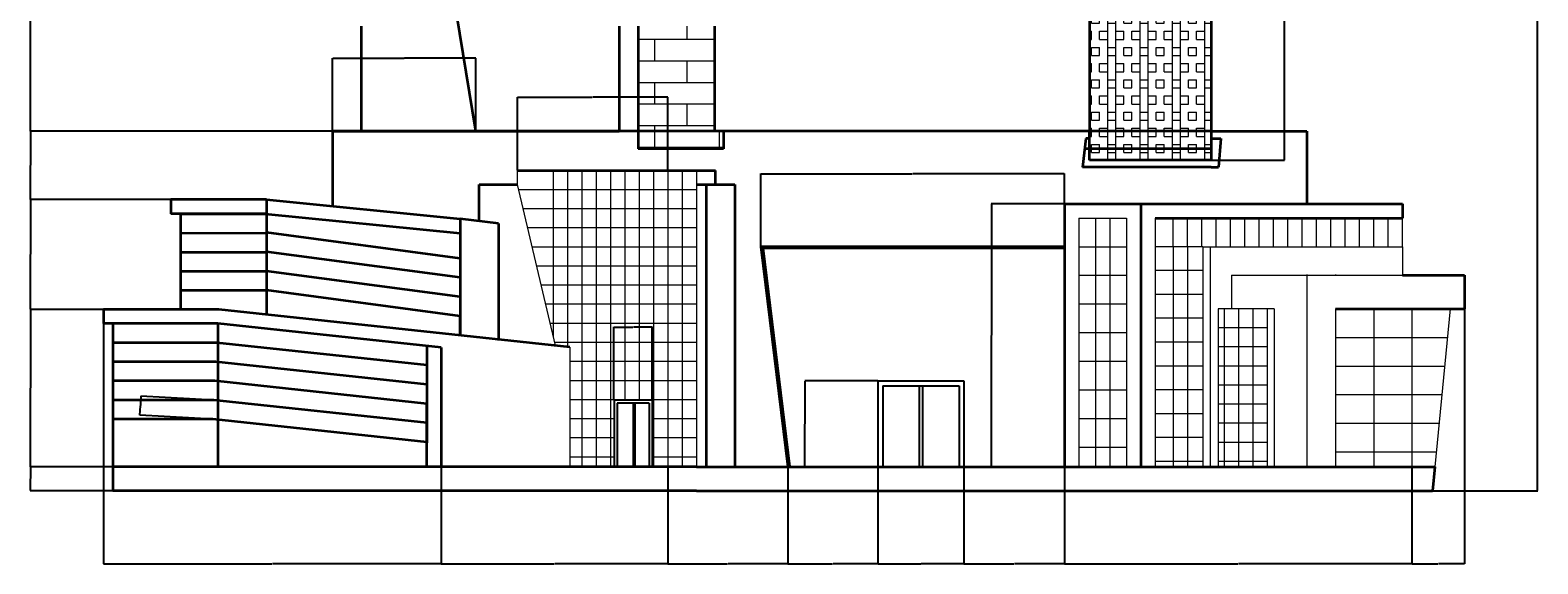
# Model space of a CAD drawing. Units: inches. Extents: x 597 to 2491, y 560 to 2558.
# Tile 1 of 2: x 597 to 2491, y 560 to 1231. Entities that reach past the tile are written whole.
import ezdxf

# ---------------------------------------------------------------- set-up
doc = ezdxf.new("R2010")
doc.units = ezdxf.units.IN
for name, color, linetype, lineweight in [('A-ANNO-DIMS', 2, 'Continuous', 18), ('A-DOOR', 3, 'Continuous', 25), ('A-ELEV', 7, 'Continuous', 35), ('A-ELEV-PATT', 8, 'Continuous', 13), ('A-GLAZ', 4, 'Continuous', 18)]:
    doc.layers.add(name, color=color, linetype=linetype, lineweight=lineweight)
doc.styles.get("Standard").update_dxf_attribs({"font": 'arial.ttf'})
doc.dimstyles.get("Standard").update_dxf_attribs({"dimtxt": 0.18, "dimasz": 0.18, "dimexe": 0.18, "dimexo": 0.0625, "dimgap": 0.09, "dimtad": 0, "dimtih": 1, "dimtoh": 1, "dimdec": 4, "dimzin": 0, "dimdsep": 46, "dimtxsty": 'Standard', "dimcen": 0.09, "dimadec": 0, "dimazin": 0, "dimtfac": 1, "dimtdec": 4, "dimtofl": 0, "dimtmove": 0, "dimatfit": 3, "dimfxl": 1, "dimtolj": 1, "dimtzin": 0, "dimarcsym": 0})

# ---------------------------------------------------------------- blocks, each defined once
blk = doc.blocks.new('*D1')
at = {"layer": 'A-ANNO-DIMS', "color": 0, "lineweight": -2, "transparency": 16777216}
for p, q in [((1478.3, 2465.8), (2491, 2465.8)), ((2490.9, 2465.6), (2490.9, 1559)), ((2490.9, 652.1), (2490.9, 1558.7)), ((701.1, 651.9), (2491, 651.9))]:
    blk.add_line(p, q, dxfattribs=at)
at = {"layer": 'A-ANNO-DIMS', "color": 0, "transparency": 16777216}
for points in [[(2490.8, 2465.6), (2490.9, 2465.6), (2490.9, 2465.8)], [(2490.8, 652.1), (2490.9, 652.1), (2490.9, 651.9)]]:
    blk.add_solid(points, dxfattribs=at)
at = {"layer": 'Defpoints', "color": 0, "transparency": 16777216}
for p in [(1478.2, 2465.8), (2490.9, 2465.8), (701, 651.9)]:
    blk.add_point(p, dxfattribs=at)
at = {"layer": 'A-ANNO-DIMS', "color": 0, "transparency": 16777216, "insert": (2490.9, 1558.9), "char_height": 0.18, "attachment_point": 5}
blk.add_mtext('\\A1;1814', dxfattribs=at)
blk = doc.blocks.new('*D2')
at = {"layer": 'A-ANNO-DIMS', "color": 0, "lineweight": -2, "transparency": 16777216}
for p, q in [((689, 861.9), (689, 560)), ((1113.3, 681.4), (1113.3, 560)), ((689.2, 560.2), (900.8, 560.2)), ((1113.1, 560.2), (901.6, 560.2))]:
    blk.add_line(p, q, dxfattribs=at)
at = {"layer": 'A-ANNO-DIMS', "color": 0, "transparency": 16777216}
for points in [[(689.2, 560.2), (689.2, 560.1), (689, 560.2)], [(1113.1, 560.2), (1113.1, 560.1), (1113.3, 560.2)]]:
    blk.add_solid(points, dxfattribs=at)
at = {"layer": 'Defpoints', "color": 0, "transparency": 16777216}
for p in [(689, 861.9), (1113.3, 681.5), (1113.3, 560.2)]:
    blk.add_point(p, dxfattribs=at)
at = {"layer": 'A-ANNO-DIMS', "color": 0, "transparency": 16777216, "insert": (901.2, 560.2), "char_height": 0.18, "attachment_point": 5}
blk.add_mtext('\\A1;424.2', dxfattribs=at)
blk = doc.blocks.new('*D3')
at = {"layer": 'A-ANNO-DIMS', "color": 0, "lineweight": -2, "transparency": 16777216}
for p, q in [((1113.3, 681.4), (1113.3, 560)), ((1398.1, 681.9), (1398.1, 560)), ((1113.4, 560.2), (1255.2, 560.2)), ((1398, 560.2), (1256.2, 560.2))]:
    blk.add_line(p, q, dxfattribs=at)
at = {"layer": 'A-ANNO-DIMS', "color": 0, "transparency": 16777216}
for points in [[(1113.4, 560.2), (1113.4, 560.1), (1113.3, 560.2)], [(1398, 560.2), (1398, 560.1), (1398.1, 560.2)]]:
    blk.add_solid(points, dxfattribs=at)
at = {"layer": 'Defpoints', "color": 0, "transparency": 16777216}
for p in [(1398.1, 681.9), (1113.3, 681.5), (1398.1, 560.2)]:
    blk.add_point(p, dxfattribs=at)
at = {"layer": 'A-ANNO-DIMS', "color": 0, "transparency": 16777216, "insert": (1255.7, 560.2), "char_height": 0.18, "attachment_point": 5}
blk.add_mtext('\\A1;284.87', dxfattribs=at)
blk = doc.blocks.new('*D4')
at = {"layer": 'A-ANNO-DIMS', "color": 0, "lineweight": -2, "transparency": 16777216}
for p, q in [((1398.1, 681.9), (1398.1, 560)), ((1548.9, 681.9), (1548.9, 560)), ((1398.3, 560.2), (1473.2, 560.2)), ((1548.8, 560.2), (1473.9, 560.2))]:
    blk.add_line(p, q, dxfattribs=at)
at = {"layer": 'A-ANNO-DIMS', "color": 0, "transparency": 16777216}
for points in [[(1398.3, 560.2), (1398.3, 560.1), (1398.1, 560.2)], [(1548.8, 560.2), (1548.8, 560.1), (1548.9, 560.2)]]:
    blk.add_solid(points, dxfattribs=at)
at = {"layer": 'Defpoints', "color": 0, "transparency": 16777216}
for p in [(1398.1, 681.9), (1548.9, 681.9), (1548.9, 560.2)]:
    blk.add_point(p, dxfattribs=at)
at = {"layer": 'A-ANNO-DIMS', "color": 0, "transparency": 16777216, "insert": (1473.5, 560.2), "char_height": 0.18, "attachment_point": 5}
blk.add_mtext('\\A1;150.8', dxfattribs=at)
blk = doc.blocks.new('*D5')
at = {"layer": 'A-ANNO-DIMS', "color": 0, "lineweight": -2, "transparency": 16777216}
for p, q in [((1548.9, 681.9), (1548.9, 560)), ((1662.1, 681.9), (1662.1, 560)), ((1549.1, 560.2), (1605.1, 560.2)), ((1661.9, 560.2), (1605.9, 560.2))]:
    blk.add_line(p, q, dxfattribs=at)
at = {"layer": 'A-ANNO-DIMS', "color": 0, "transparency": 16777216}
for points in [[(1549.1, 560.2), (1549.1, 560.1), (1548.9, 560.2)], [(1661.9, 560.2), (1661.9, 560.1), (1662.1, 560.2)]]:
    blk.add_solid(points, dxfattribs=at)
at = {"layer": 'Defpoints', "color": 0, "transparency": 16777216}
for p in [(1548.9, 681.9), (1662.1, 681.9), (1662.1, 560.2)]:
    blk.add_point(p, dxfattribs=at)
at = {"layer": 'A-ANNO-DIMS', "color": 0, "transparency": 16777216, "insert": (1605.5, 560.2), "char_height": 0.18, "attachment_point": 5}
blk.add_mtext('\\A1;113.1', dxfattribs=at)
blk = doc.blocks.new('*D6')
at = {"layer": 'A-ANNO-DIMS', "color": 0, "lineweight": -2, "transparency": 16777216}
for p, q in [((1662.1, 681.9), (1662.1, 560)), ((1770.1, 681.9), (1770.1, 560)), ((1662.2, 560.2), (1715.8, 560.2)), ((1769.9, 560.2), (1716.3, 560.2))]:
    blk.add_line(p, q, dxfattribs=at)
at = {"layer": 'A-ANNO-DIMS', "color": 0, "transparency": 16777216}
for points in [[(1662.2, 560.2), (1662.2, 560.1), (1662.1, 560.2)], [(1769.9, 560.2), (1769.9, 560.1), (1770.1, 560.2)]]:
    blk.add_solid(points, dxfattribs=at)
at = {"layer": 'Defpoints', "color": 0, "transparency": 16777216}
for p in [(1662.1, 681.9), (1770.1, 681.9), (1770.1, 560.2)]:
    blk.add_point(p, dxfattribs=at)
at = {"layer": 'A-ANNO-DIMS', "color": 0, "transparency": 16777216, "insert": (1716.1, 560.2), "char_height": 0.18, "attachment_point": 5}
blk.add_mtext('\\A1;108', dxfattribs=at)
blk = doc.blocks.new('*D7')
at = {"layer": 'A-ANNO-DIMS', "color": 0, "lineweight": -2, "transparency": 16777216}
for p, q in [((1770.1, 681.9), (1770.1, 560)), ((1896.4, 681.9), (1896.4, 560)), ((1770.2, 560.2), (1832.8, 560.2)), ((1896.2, 560.2), (1833.7, 560.2))]:
    blk.add_line(p, q, dxfattribs=at)
at = {"layer": 'A-ANNO-DIMS', "color": 0, "transparency": 16777216}
for points in [[(1770.2, 560.2), (1770.2, 560.1), (1770.1, 560.2)], [(1896.2, 560.2), (1896.2, 560.1), (1896.4, 560.2)]]:
    blk.add_solid(points, dxfattribs=at)
at = {"layer": 'Defpoints', "color": 0, "transparency": 16777216}
for p in [(1770.1, 681.9), (1896.4, 681.9), (1896.4, 560.2)]:
    blk.add_point(p, dxfattribs=at)
at = {"layer": 'A-ANNO-DIMS', "color": 0, "transparency": 16777216, "insert": (1833.2, 560.2), "char_height": 0.18, "attachment_point": 5}
blk.add_mtext('\\A1;126.33', dxfattribs=at)
blk = doc.blocks.new('*D8')
at = {"layer": 'A-ANNO-DIMS', "color": 0, "lineweight": -2, "transparency": 16777216}
for p, q in [((1896.4, 681.9), (1896.4, 560)), ((2332.9, 681.9), (2332.9, 560)), ((1896.6, 560.2), (2114.3, 560.2)), ((2332.8, 560.2), (2115.1, 560.2))]:
    blk.add_line(p, q, dxfattribs=at)
at = {"layer": 'A-ANNO-DIMS', "color": 0, "transparency": 16777216}
for points in [[(1896.6, 560.2), (1896.6, 560.1), (1896.4, 560.2)], [(2332.8, 560.2), (2332.8, 560.1), (2332.9, 560.2)]]:
    blk.add_solid(points, dxfattribs=at)
at = {"layer": 'Defpoints', "color": 0, "transparency": 16777216}
for p in [(1896.4, 681.9), (2332.9, 681.9), (2332.9, 560.2)]:
    blk.add_point(p, dxfattribs=at)
at = {"layer": 'A-ANNO-DIMS', "color": 0, "transparency": 16777216, "insert": (2114.7, 560.2), "char_height": 0.18, "attachment_point": 5}
blk.add_mtext('\\A1;436.6', dxfattribs=at)
blk = doc.blocks.new('*D9')
at = {"layer": 'A-ANNO-DIMS', "color": 0, "lineweight": -2, "transparency": 16777216}
for p, q in [((2399.1, 880.6), (2399.1, 560)), ((2332.9, 681.9), (2332.9, 560)), ((2333.1, 560.2), (2365.6, 560.2)), ((2398.9, 560.2), (2366.4, 560.2))]:
    blk.add_line(p, q, dxfattribs=at)
at = {"layer": 'A-ANNO-DIMS', "color": 0, "transparency": 16777216}
for points in [[(2333.1, 560.2), (2333.1, 560.1), (2332.9, 560.2)], [(2398.9, 560.2), (2398.9, 560.1), (2399.1, 560.2)]]:
    blk.add_solid(points, dxfattribs=at)
at = {"layer": 'Defpoints', "color": 0, "transparency": 16777216}
for p in [(2399.1, 880.7), (2332.9, 681.9), (2399.1, 560.2)]:
    blk.add_point(p, dxfattribs=at)
at = {"layer": 'A-ANNO-DIMS', "color": 0, "transparency": 16777216, "insert": (2366, 560.2), "char_height": 0.18, "attachment_point": 5}
blk.add_mtext('\\A1;66.18', dxfattribs=at)
blk = doc.blocks.new('*D15')
at = {"layer": 'A-ANNO-DIMS', "color": 0, "lineweight": -2, "transparency": 16777216}
for p, q in [((701, 681.9), (597.1, 681.9)), ((597.3, 681.7), (597.3, 667.1)), ((597.3, 652.1), (597.3, 666.7)), ((701, 651.9), (597.1, 651.9))]:
    blk.add_line(p, q, dxfattribs=at)
at = {"layer": 'A-ANNO-DIMS', "color": 0, "transparency": 16777216}
for points in [[(597.3, 681.7), (597.3, 681.7), (597.3, 681.9)], [(597.3, 652.1), (597.3, 652.1), (597.3, 651.9)]]:
    blk.add_solid(points, dxfattribs=at)
at = {"layer": 'Defpoints', "color": 0, "transparency": 16777216}
for p in [(597.3, 681.9), (701, 681.9), (701, 651.9)]:
    blk.add_point(p, dxfattribs=at)
at = {"layer": 'A-ANNO-DIMS', "color": 0, "transparency": 16777216, "insert": (597.3, 666.9), "char_height": 0.18, "attachment_point": 5}
blk.add_mtext('\\A1;30', dxfattribs=at)
blk = doc.blocks.new('*D16')
at = {"layer": 'A-ANNO-DIMS', "color": 0, "lineweight": -2, "transparency": 16777216}
for p, q in [((689, 879.9), (597.1, 879.9)), ((597.3, 879.7), (597.3, 781.1)), ((597.3, 682.1), (597.3, 780.7)), ((701, 681.9), (597.1, 681.9))]:
    blk.add_line(p, q, dxfattribs=at)
at = {"layer": 'A-ANNO-DIMS', "color": 0, "transparency": 16777216}
for points in [[(597.3, 879.7), (597.3, 879.7), (597.3, 879.9)], [(597.3, 682.1), (597.3, 682.1), (597.3, 681.9)]]:
    blk.add_solid(points, dxfattribs=at)
at = {"layer": 'Defpoints', "color": 0, "transparency": 16777216}
for p in [(597.3, 879.9), (689, 879.9), (701, 681.9)]:
    blk.add_point(p, dxfattribs=at)
at = {"layer": 'A-ANNO-DIMS', "color": 0, "transparency": 16777216, "insert": (597.3, 780.9), "char_height": 0.18, "attachment_point": 5}
blk.add_mtext('\\A1;198', dxfattribs=at)
blk = doc.blocks.new('*D17')
at = {"layer": 'A-ANNO-DIMS', "color": 0, "lineweight": -2, "transparency": 16777216}
for p, q in [((773.9, 1017.9), (597.1, 1017.9)), ((597.3, 1017.7), (597.3, 949.1)), ((597.3, 880.1), (597.3, 948.7)), ((689, 879.9), (597.1, 879.9))]:
    blk.add_line(p, q, dxfattribs=at)
at = {"layer": 'A-ANNO-DIMS', "color": 0, "transparency": 16777216}
for points in [[(597.3, 1017.7), (597.3, 1017.7), (597.3, 1017.9)], [(597.3, 880.1), (597.3, 880.1), (597.3, 879.9)]]:
    blk.add_solid(points, dxfattribs=at)
at = {"layer": 'Defpoints', "color": 0, "transparency": 16777216}
for p in [(597.3, 1017.9), (773.9, 1017.9), (689, 879.9)]:
    blk.add_point(p, dxfattribs=at)
at = {"layer": 'A-ANNO-DIMS', "color": 0, "transparency": 16777216, "insert": (597.3, 948.9), "char_height": 0.18, "attachment_point": 5}
blk.add_mtext('\\A1;138', dxfattribs=at)
blk = doc.blocks.new('*D18')
at = {"layer": 'A-ANNO-DIMS', "color": 0, "lineweight": -2, "transparency": 16777216}
for p, q in [((976.9, 1103.8), (597.1, 1103.8)), ((597.3, 1103.6), (597.3, 1061)), ((597.3, 1018.1), (597.3, 1060.7)), ((773.9, 1017.9), (597.1, 1017.9))]:
    blk.add_line(p, q, dxfattribs=at)
at = {"layer": 'A-ANNO-DIMS', "color": 0, "transparency": 16777216}
for points in [[(597.3, 1103.6), (597.3, 1103.6), (597.3, 1103.8)], [(597.3, 1018.1), (597.3, 1018.1), (597.3, 1017.9)]]:
    blk.add_solid(points, dxfattribs=at)
at = {"layer": 'Defpoints', "color": 0, "transparency": 16777216}
for p in [(597.3, 1103.8), (976.9, 1103.8), (773.9, 1017.9)]:
    blk.add_point(p, dxfattribs=at)
at = {"layer": 'A-ANNO-DIMS', "color": 0, "transparency": 16777216, "insert": (597.3, 1060.9), "char_height": 0.18, "attachment_point": 5}
blk.add_mtext('\\A1;85.9', dxfattribs=at)
blk = doc.blocks.new('*D19')
at = {"layer": 'A-ANNO-DIMS', "color": 0, "lineweight": -2, "transparency": 16777216}
for p, q in [((976.9, 2207.8), (597.1, 2207.8)), ((597.3, 2207.6), (597.3, 1656)), ((597.3, 1104), (597.3, 1655.6)), ((976.9, 1103.8), (597.1, 1103.8))]:
    blk.add_line(p, q, dxfattribs=at)
at = {"layer": 'A-ANNO-DIMS', "color": 0, "transparency": 16777216}
for points in [[(597.3, 2207.6), (597.3, 2207.6), (597.3, 2207.8)], [(597.3, 1104), (597.3, 1104), (597.3, 1103.8)]]:
    blk.add_solid(points, dxfattribs=at)
at = {"layer": 'Defpoints', "color": 0, "transparency": 16777216}
for p in [(597.3, 2207.8), (976.9, 2207.8), (976.9, 1103.8)]:
    blk.add_point(p, dxfattribs=at)
at = {"layer": 'A-ANNO-DIMS', "color": 0, "transparency": 16777216, "insert": (597.3, 1655.8), "char_height": 0.18, "attachment_point": 5}
blk.add_mtext('\\A1;1104', dxfattribs=at)
blk = doc.blocks.new('*D24')
at = {"layer": 'A-ANNO-DIMS', "color": 0, "lineweight": -2, "transparency": 16777216}
for p, q in [((1662, 789.9), (1570.1, 789.9)), ((1570.3, 789.7), (1570.3, 736.1)), ((1570.3, 682.1), (1570.3, 735.7)), ((1662, 681.9), (1570.1, 681.9))]:
    blk.add_line(p, q, dxfattribs=at)
at = {"layer": 'A-ANNO-DIMS', "color": 0, "transparency": 16777216}
for points in [[(1570.3, 789.7), (1570.3, 789.7), (1570.3, 789.9)], [(1570.3, 682.1), (1570.3, 682.1), (1570.3, 681.9)]]:
    blk.add_solid(points, dxfattribs=at)
at = {"layer": 'Defpoints', "color": 0, "transparency": 16777216}
for p in [(1570.3, 789.9), (1662.1, 789.9), (1662.1, 681.9)]:
    blk.add_point(p, dxfattribs=at)
at = {"layer": 'A-ANNO-DIMS', "color": 0, "transparency": 16777216, "insert": (1570.3, 735.9), "char_height": 0.18, "attachment_point": 5}
blk.add_mtext('\\A1;108', dxfattribs=at)
blk = doc.blocks.new('*D25')
at = {"layer": 'A-ANNO-DIMS', "color": 0, "lineweight": -2, "transparency": 16777216}
for p, q in [((1896.3, 1012.7), (1804.5, 1012.7)), ((1804.6, 1012.5), (1804.6, 847.5)), ((1804.6, 682.1), (1804.6, 847.1)), ((1896.3, 681.9), (1804.5, 681.9))]:
    blk.add_line(p, q, dxfattribs=at)
at = {"layer": 'A-ANNO-DIMS', "color": 0, "transparency": 16777216}
for points in [[(1804.6, 1012.5), (1804.7, 1012.5), (1804.6, 1012.7)], [(1804.6, 682.1), (1804.7, 682.1), (1804.6, 681.9)]]:
    blk.add_solid(points, dxfattribs=at)
at = {"layer": 'Defpoints', "color": 0, "transparency": 16777216}
for p in [(1804.6, 1012.7), (1896.4, 1012.7), (1896.4, 681.9)]:
    blk.add_point(p, dxfattribs=at)
at = {"layer": 'A-ANNO-DIMS', "color": 0, "transparency": 16777216, "insert": (1804.6, 847.3), "char_height": 0.18, "attachment_point": 5}
blk.add_mtext('\\A1;330.76', dxfattribs=at)
blk = doc.blocks.new('*D26')
at = {"layer": 'A-ANNO-DIMS', "color": 0, "lineweight": -2, "transparency": 16777216}
for p, q in [((1515.1, 958.7), (1515.1, 1050.6)), ((1515.2, 1050.4), (1705.3, 1050.4)), ((1896.2, 1050.4), (1706.1, 1050.4)), ((1896.4, 958.7), (1896.4, 1050.6))]:
    blk.add_line(p, q, dxfattribs=at)
at = {"layer": 'A-ANNO-DIMS', "color": 0, "transparency": 16777216}
for points in [[(1515.2, 1050.4), (1515.2, 1050.4), (1515.1, 1050.4)], [(1896.2, 1050.4), (1896.2, 1050.4), (1896.4, 1050.4)]]:
    blk.add_solid(points, dxfattribs=at)
at = {"layer": 'Defpoints', "color": 0, "transparency": 16777216}
for p in [(1896.4, 1050.4), (1515.1, 958.7), (1896.4, 958.7)]:
    blk.add_point(p, dxfattribs=at)
at = {"layer": 'A-ANNO-DIMS', "color": 0, "transparency": 16777216, "insert": (1705.7, 1050.4), "char_height": 0.18, "attachment_point": 5}
blk.add_mtext('\\A1;381.3', dxfattribs=at)
blk = doc.blocks.new('*D27')
at = {"layer": 'A-ANNO-DIMS', "color": 0, "lineweight": -2, "transparency": 16777216}
for p, q in [((976.9, 1103.9), (976.9, 1195.7)), ((977.1, 1195.6), (1066.7, 1195.6)), ((1156.8, 1195.6), (1067.2, 1195.6)), ((1156.9, 1103.9), (1156.9, 1195.7))]:
    blk.add_line(p, q, dxfattribs=at)
at = {"layer": 'A-ANNO-DIMS', "color": 0, "transparency": 16777216}
for points in [[(977.1, 1195.6), (977.1, 1195.5), (976.9, 1195.6)], [(1156.8, 1195.6), (1156.8, 1195.5), (1156.9, 1195.6)]]:
    blk.add_solid(points, dxfattribs=at)
at = {"layer": 'Defpoints', "color": 0, "transparency": 16777216}
for p in [(1156.9, 1195.6), (976.9, 1103.8), (1156.9, 1103.8)]:
    blk.add_point(p, dxfattribs=at)
at = {"layer": 'A-ANNO-DIMS', "color": 0, "transparency": 16777216, "insert": (1066.9, 1195.6), "char_height": 0.18, "attachment_point": 5}
blk.add_mtext('\\A1;180', dxfattribs=at)
blk = doc.blocks.new('*D32')
at = {"layer": 'A-ANNO-DIMS', "color": 0, "lineweight": -2, "transparency": 16777216}
for p, q in [((2081, 2183.8), (2172.9, 2183.8)), ((2172.7, 2183.6), (2172.7, 1625.8)), ((2172.7, 1067.6), (2172.7, 1625.4)), ((2081, 1067.4), (2172.9, 1067.4))]:
    blk.add_line(p, q, dxfattribs=at)
at = {"layer": 'A-ANNO-DIMS', "color": 0, "transparency": 16777216}
for points in [[(2172.7, 2183.6), (2172.7, 2183.6), (2172.7, 2183.8)], [(2172.7, 1067.6), (2172.7, 1067.6), (2172.7, 1067.4)]]:
    blk.add_solid(points, dxfattribs=at)
at = {"layer": 'Defpoints', "color": 0, "transparency": 16777216}
for p in [(2080.9, 2183.8), (2080.9, 1067.4), (2172.7, 1067.4)]:
    blk.add_point(p, dxfattribs=at)
at = {"layer": 'A-ANNO-DIMS', "color": 0, "transparency": 16777216, "insert": (2172.7, 1625.6), "char_height": 0.18, "attachment_point": 5}
blk.add_mtext('\\A1;1116.4', dxfattribs=at)
blk = doc.blocks.new('*D36')
at = {"layer": 'A-ANNO-DIMS', "color": 0, "lineweight": -2, "transparency": 16777216}
for p, q in [((1209.1, 1054.7), (1209.1, 1146.6)), ((1209.3, 1146.4), (1303.2, 1146.4)), ((1398, 1146.4), (1304.1, 1146.4)), ((1398.1, 1054.7), (1398.1, 1146.6))]:
    blk.add_line(p, q, dxfattribs=at)
at = {"layer": 'A-ANNO-DIMS', "color": 0, "transparency": 16777216}
for points in [[(1209.3, 1146.4), (1209.3, 1146.4), (1209.1, 1146.4)], [(1398, 1146.4), (1398, 1146.4), (1398.1, 1146.4)]]:
    blk.add_solid(points, dxfattribs=at)
at = {"layer": 'Defpoints', "color": 0, "transparency": 16777216}
for p in [(1398.1, 1146.4), (1209.1, 1054.6), (1398.1, 1054.6)]:
    blk.add_point(p, dxfattribs=at)
at = {"layer": 'A-ANNO-DIMS', "color": 0, "transparency": 16777216, "insert": (1303.6, 1146.4), "char_height": 0.18, "attachment_point": 5}
blk.add_mtext('\\A1;189.04', dxfattribs=at)
blk = doc.blocks.new('*D37')
at = {"layer": 'A-ANNO-DIMS', "color": 0, "lineweight": -2, "transparency": 16777216}
for p, q in [((1330.5, 766), (1330.5, 857.8)), ((1330.7, 857.7), (1354.3, 857.7)), ((1378.4, 857.7), (1354.8, 857.7)), ((1378.5, 766), (1378.5, 857.8))]:
    blk.add_line(p, q, dxfattribs=at)
at = {"layer": 'A-ANNO-DIMS', "color": 0, "transparency": 16777216}
for points in [[(1330.7, 857.7), (1330.7, 857.6), (1330.5, 857.7)], [(1378.4, 857.7), (1378.4, 857.6), (1378.5, 857.7)]]:
    blk.add_solid(points, dxfattribs=at)
at = {"layer": 'Defpoints', "color": 0, "transparency": 16777216}
for p in [(1378.5, 857.7), (1330.5, 765.9), (1378.5, 765.9)]:
    blk.add_point(p, dxfattribs=at)
at = {"layer": 'A-ANNO-DIMS', "color": 0, "transparency": 16777216, "insert": (1354.5, 857.7), "char_height": 0.18, "attachment_point": 5}
blk.add_mtext('\\A1;48', dxfattribs=at)
blk = doc.blocks.new('*D38')
at = {"layer": 'A-ANNO-DIMS', "color": 0, "lineweight": -2, "transparency": 16777216}
for p, q in [((734.9, 747), (735.6, 758.6)), ((736.2, 770.6), (735.6, 759)), ((827.8, 765.9), (736, 770.8)), ((826.5, 741.9), (734.8, 746.8))]:
    blk.add_line(p, q, dxfattribs=at)
at = {"layer": 'A-ANNO-DIMS', "color": 0, "transparency": 16777216}
for points in [[(736.2, 770.6), (736.2, 770.6), (736.2, 770.8)], [(734.9, 747), (735, 747), (734.9, 746.8)]]:
    blk.add_solid(points, dxfattribs=at)
at = {"layer": 'Defpoints', "color": 0, "transparency": 16777216}
for p in [(736.2, 770.8), (827.8, 765.9), (826.5, 741.9)]:
    blk.add_point(p, dxfattribs=at)
at = {"layer": 'A-ANNO-DIMS', "color": 0, "transparency": 16777216, "insert": (735.6, 758.8), "char_height": 0.18, "attachment_point": 5}
blk.add_mtext('\\A1;24.034', dxfattribs=at)

msp = doc.modelspace()

# ---------------------------------------------------------------- hatches: boundary and pattern name
at = {"layer": 'A-ELEV-PATT'}
h = msp.add_hatch(dxfattribs=at)
h.set_pattern_fill('BOX', color=256, scale=1.6)
h.paths.add_polyline_path([(2080.9409, 2183.8154), (1987.9409, 2183.8154), (1987.9409, 1433.8154), (1987.9409, 1373.8154), (1927.9409, 1373.8154), (1927.9409, 1253.8154), (1927.9409, 1103.8154), (2080.9409, 1103.8154)])
h = msp.add_hatch(dxfattribs=at)
h.set_pattern_fill('AR-BRSTD', color=256, scale=0.4)
h.paths.add_polyline_path([(1927.9409, 2165.8154), (1360.9409, 2165.8154), (1360.9409, 2081.8154), (1927.9409, 2081.8154)])
h.paths.add_polyline_path([(1456.9409, 2081.8154), (1360.9409, 2081.8154), (1360.9409, 1985.8154), (1456.9409, 1985.8154)])
h.paths.add_polyline_path([(1456.9409, 1925.8154), (1360.9409, 1925.8154), (1360.9409, 1847.8154), (1456.9409, 1847.8154)])
h.paths.add_polyline_path([(1456.9409, 1787.8154), (1360.9409, 1787.8154), (1360.9409, 1709.8154), (1456.9409, 1709.8154)])
h.paths.add_polyline_path([(1456.9409, 1649.8154), (1360.9409, 1649.8154), (1360.9409, 1571.8154), (1456.9409, 1571.8154)])
h.paths.add_polyline_path([(1456.9409, 1511.8154), (1360.9409, 1511.8154), (1360.9409, 1433.8154), (1456.9409, 1433.8154)])
h.paths.add_polyline_path([(1456.9409, 1373.8154), (1360.9409, 1373.8154), (1360.9409, 1295.8154), (1456.9409, 1295.8154)])
h.paths.add_polyline_path([(1456.9409, 1235.8154), (1360.9409, 1235.8154), (1360.9409, 1103.8154), (1456.9409, 1103.8154)])
h = msp.add_hatch(dxfattribs=at)
h.set_pattern_fill('AR-BRSTD', color=256, scale=0.4)
h.paths.add_polyline_path([(1467.9409, 1103.8154), (1360.9409, 1103.8154), (1360.9409, 1081.8154), (1467.9409, 1081.8154)])
h = msp.add_hatch(dxfattribs=at)
h.set_pattern_fill('BOX', color=256, scale=1.6)
h.paths.add_polyline_path([(2080.9409, 1103.8154), (1927.9409, 1103.8154), (1927.9409, 1067.4311), (2080.9409, 1067.4311)])

# ---------------------------------------------------------------- linework, layer by layer
at = {"layer": 'A-DOOR'}
for p, q in [((1662.0507, 789.9147), (1770.0507, 789.9147)), ((1662.0507, 789.9147), (1662.0507, 681.9147)), ((1668.0507, 783.9147), (1668.0507, 681.9147)), ((1668.0507, 783.9147), (1764.0507, 783.9147)), ((1714.0507, 783.9147), (1714.0507, 681.9147)), ((1718.0507, 783.9147), (1718.0507, 681.9147)), ((1764.0507, 783.9147), (1764.0507, 681.9147)), ((1770.0507, 789.9147), (1770.0507, 681.9147)), ((1330.534, 765.9147), (1330.534, 681.9147)), ((1378.534, 765.9147), (1330.534, 765.9147)), ((1334.534, 761.9147), (1334.534, 681.9147)), ((1374.534, 761.9147), (1334.534, 761.9147)), ((1354.534, 761.9147), (1354.534, 681.9147)), ((1355.534, 761.9147), (1355.534, 681.9147)), ((1356.534, 761.9147), (1356.534, 681.9147)), ((1374.534, 761.9147), (1374.534, 681.9147)), ((1378.534, 765.9147), (1378.534, 681.9147))]:
    msp.add_line(p, q, dxfattribs=at)
at = {"layer": 'A-ELEV'}
for p, q in [((1156.9409, 1103.8154), (976.9409, 2207.8154)), ((2080.9409, 2183.8154), (2080.9409, 1103.8154)), ((1927.9409, 1253.8154), (1927.9409, 1103.8154)), ((1012.9409, 1235.8154), (1012.9409, 1103.8154)), ((1336.9409, 1235.8154), (1336.9409, 1103.8154)), ((1360.9409, 1235.8154), (1360.9409, 1081.8154)), ((1456.9409, 1235.8154), (1456.9409, 1103.8154)), ((2080.9409, 1103.8154), (976.9409, 1103.8154)), ((976.9409, 1103.8154), (1336.9409, 1103.8154)), ((976.9409, 1103.8154), (976.9409, 1009.673)), ((1467.9409, 1103.8154), (1467.9409, 1081.8154)), ((1927.9409, 1067.4311), (1927.9409, 1103.8154)), ((2080.9409, 1103.8154), (2200.9409, 1103.8154)), ((2080.9409, 1103.8154), (2080.9409, 1067.4311)), ((2200.9409, 1103.8154), (2200.9409, 1012.6753)), ((1467.9409, 1081.8154), (1360.9409, 1081.8154)), ((1923.4409, 1094.8154), (1918.9409, 1058.4311)), ((2080.9409, 1081.8154), (1921.833, 1081.8154)), ((1927.9409, 1094.8154), (1923.4409, 1094.8154)), ((2080.9409, 1094.8154), (2092.9409, 1094.8154)), ((2089.9409, 1094.8154), (2092.9409, 1094.8154)), ((2092.9409, 1094.8154), (2089.9409, 1058.4311)), ((2080.9409, 1067.4311), (1927.9409, 1067.4311)), ((1209.0993, 1054.6363), (1458.1392, 1054.6363)), ((1458.1392, 1036.6363), (1458.1392, 1054.6363)), ((1927.9409, 1058.4311), (1918.9409, 1058.4311)), ((2080.9409, 1058.4311), (1927.9409, 1058.4311)), ((2080.9409, 1058.4311), (2089.9409, 1058.4311)), ((1161.2698, 990.7733), (1161.2698, 1036.9434)), ((1161.2698, 1036.9434), (1209.0993, 1036.9434)), ((1434.1392, 1036.6363), (1482.1392, 1036.6363)), ((1446.1392, 1036.6363), (1446.1392, 681.9147)), ((1482.1392, 1036.6363), (1482.1392, 681.9147)), ((893.9426, 1017.9147), (773.9426, 1017.9147)), ((773.9426, 1017.9147), (773.9426, 999.9147)), ((893.9426, 1017.9147), (893.9426, 873.4666)), ((893.9426, 1017.9147), (1137.2698, 993.7523)), ((1896.3835, 1012.6753), (1896.3835, 681.9147)), ((1896.3835, 1012.6753), (2320.9409, 1012.6753)), ((1992.3835, 1012.6753), (1992.3835, 681.9147)), ((2320.9409, 1012.6753), (2320.9409, 994.6753)), ((893.9426, 999.9147), (773.9426, 999.9147)), ((785.9426, 999.9147), (785.9426, 879.9147)), ((785.9426, 999.9147), (893.9426, 999.8262)), ((892.164, 1000.0028), (1137.2698, 975.6638)), ((1137.2698, 993.7523), (1137.2698, 847.3169)), ((1185.2698, 987.7943), (1137.2698, 993.7523)), ((1185.2698, 987.7943), (1185.2698, 840.8688)), ((2010.3835, 994.6753), (2320.9409, 994.6753)), ((785.923, 975.9147), (893.923, 975.8262)), ((1137.2698, 943.9562), (893.9426, 976.455)), ((785.9033, 951.9147), (893.9033, 951.8262)), ((1137.2698, 919.7431), (893.9426, 952.2419)), ((1896.3835, 958.6532), (1515.0557, 958.6532)), ((1515.0557, 958.6532), (1548.9426, 681.9147)), ((1896.3835, 956.6532), (1517.3156, 956.6532)), ((1517.3156, 956.6532), (1550.9278, 682.1578)), ((785.8836, 927.9147), (893.8836, 927.8262)), ((1137.2698, 895.53), (893.9426, 928.0288)), ((2320.9409, 922.6753), (2399.1184, 922.6753)), ((2399.1184, 922.6753), (2399.1184, 880.6753)), ((785.8639, 903.9147), (893.8639, 903.8262)), ((1137.2698, 871.3169), (893.8639, 903.8262)), ((689.0424, 879.9147), (689.0424, 861.9147)), ((1137.2698, 847.3169), (1137.2698, 871.3169)), ((2236.9409, 880.6753), (2399.1184, 880.6753)), ((701.0424, 861.9147), (701.0424, 681.9147)), ((832.9782, 861.9147), (832.9782, 681.9147)), ((1095.2698, 833.7269), (1095.2698, 711.9147)), ((1113.2698, 831.7924), (1113.2698, 711.9147)), ((1535.7179, 783.9147), (1536.4526, 783.9147)), ((1095.2698, 681.9147), (1095.2698, 761.3123)), ((1095.2698, 743.2086), (1095.2698, 727.7275)), ((1113.2698, 711.9147), (1113.2698, 681.4843)), ((1434.1392, 681.9147), (701.0424, 681.9147)), ((701.0424, 681.9147), (701.0424, 651.9147)), ((1434.1392, 681.9147), (2361.8459, 681.9147)), ((2361.8459, 681.9147), (2358.9255, 651.9147)), ((1434.1392, 651.9147), (701.0424, 651.9147)), ((1434.1392, 651.9147), (2358.9255, 651.9147))]:
    msp.add_line(p, q, dxfattribs=at)
for points in [[(1274.9288, 832.523), (833.9426, 879.9147), (773.9426, 879.9147), (689.0424, 879.9147)], [(1113.2698, 831.7924), (832.9782, 861.9147), (773.9426, 861.9147), (689.0424, 861.9147)], [(1095.2698, 809.5887), (831.6923, 837.9147), (773.9426, 837.9147), (701.0424, 837.9147)], [(1095.2698, 785.4505), (830.4064, 813.9147), (773.9426, 813.9147), (701.0424, 813.9147)], [(1095.2698, 761.3123), (829.1205, 789.9147), (773.9426, 789.9147), (701.0424, 789.9147)], [(1095.2698, 737.1741), (827.8346, 765.9147), (773.9426, 765.9147), (701.0424, 765.9147)], [(1095.2698, 713.0359), (826.5487, 741.9147), (773.9426, 741.9147), (701.0424, 741.9147)]]:
    msp.add_lwpolyline(points, dxfattribs=at)
at = {"layer": 'A-GLAZ'}
for p, q in [((1209.0993, 1036.9434), (1209.0993, 1054.6363)), ((1254.1392, 1054.6363), (1254.1392, 846.2673)), ((1272.1392, 1054.6363), (1272.1392, 832.8228)), ((1290.1392, 1054.6363), (1290.1392, 681.9147)), ((1308.1392, 1054.6363), (1308.1392, 681.9147)), ((1326.1392, 1054.6363), (1326.1392, 681.9147)), ((1344.1392, 1054.6363), (1344.1392, 765.9147)), ((1362.1392, 1054.6363), (1362.1392, 765.9147)), ((1380.1392, 1054.6363), (1380.1392, 681.9147)), ((1398.1392, 1054.6363), (1398.1392, 681.9147)), ((1416.1392, 1054.6363), (1416.1392, 681.9147)), ((1434.1392, 1054.6363), (1434.1392, 681.9147)), ((1256.9288, 834.4574), (1209.0993, 1036.9434)), ((1209.0993, 1036.6363), (1209.1719, 1036.6363)), ((1210.5891, 1030.6363), (1434.1392, 1030.6363)), ((1216.2582, 1006.6363), (1434.1392, 1006.6363)), ((1914.3835, 994.6753), (1974.3835, 994.6753)), ((1914.3835, 994.6753), (1914.3835, 681.9147)), ((1935.3835, 994.6753), (1935.3835, 681.9147)), ((1953.3835, 994.6753), (1953.3835, 681.9147)), ((1974.3835, 994.6753), (1974.3835, 681.9147)), ((2010.3835, 994.6753), (2010.3835, 681.9147)), ((2032.9409, 958.6753), (2032.9409, 994.6753)), ((2050.9409, 958.6753), (2050.9409, 994.6753)), ((2068.9409, 958.6753), (2068.9409, 994.6753)), ((2086.9409, 958.6753), (2086.9409, 994.6753)), ((2104.9409, 958.6753), (2104.9409, 994.6753)), ((2122.9409, 958.6753), (2122.9409, 994.6753)), ((2140.9409, 958.6753), (2140.9409, 994.6753)), ((2158.9409, 958.6753), (2158.9409, 994.6753)), ((2176.9409, 958.6753), (2176.9409, 994.6753)), ((2194.9409, 958.6753), (2194.9409, 994.6753)), ((2212.9409, 958.6753), (2212.9409, 994.6753)), ((2230.9409, 958.6753), (2230.9409, 994.6753)), ((2248.9409, 958.6753), (2248.9409, 994.6753)), ((2266.9409, 958.6753), (2266.9409, 994.6753)), ((2284.9409, 958.6753), (2284.9409, 994.6753)), ((2302.9409, 958.6753), (2302.9409, 994.6753)), ((2320.9409, 994.6753), (2308.9409, 994.6753)), ((2320.9409, 958.6753), (2320.9409, 994.6753)), ((1221.9273, 982.6363), (1434.1392, 982.6363)), ((1227.5964, 958.6363), (1434.1392, 958.6363)), ((1914.3835, 958.6753), (1974.3835, 958.6753)), ((2070.3835, 958.6753), (2010.3835, 958.6753)), ((2032.9409, 958.6753), (2032.9409, 681.9147)), ((2050.9409, 958.6753), (2050.9409, 681.9147)), ((2070.3835, 958.6753), (2320.9409, 958.6753)), ((2070.3835, 958.6753), (2070.3835, 681.9147)), ((2079.3835, 958.6753), (2079.3835, 681.9147)), ((2320.9409, 958.6753), (2320.9409, 922.6753)), ((1233.2654, 934.6363), (1434.1392, 934.6363)), ((2070.3835, 928.6753), (2010.3835, 928.6753)), ((1238.9345, 910.6363), (1434.1392, 910.6363)), ((1914.3835, 922.6753), (1974.3835, 922.6753)), ((2106.3835, 922.6753), (2320.9409, 922.6753)), ((2106.3835, 922.6753), (2106.3835, 880.6753)), ((2200.9409, 923.8154), (2200.9409, 681.9147)), ((2236.9409, 923.8154), (2236.9409, 922.6753)), ((2070.3835, 898.6753), (2010.3835, 898.6753)), ((1244.6036, 886.6363), (1434.1392, 886.6363)), ((1914.3835, 886.6753), (1974.3835, 886.6753)), ((2159.9413, 880.6753), (2089.4909, 880.6753)), ((2089.4909, 880.6753), (2089.4909, 681.9147)), ((2096.9413, 880.6753), (2096.9413, 681.9147)), ((2114.9413, 880.6753), (2114.9413, 681.9147)), ((2132.9413, 880.6753), (2132.9413, 681.9147)), ((2150.9413, 880.6753), (2150.9413, 681.9147)), ((2159.9413, 880.6753), (2159.9413, 681.9147)), ((2236.9409, 880.6753), (2236.9409, 681.9147)), ((2284.9409, 880.6753), (2284.9409, 681.9147)), ((2332.9409, 880.6753), (2332.9409, 681.9147)), ((2381.1942, 880.6753), (2361.8459, 681.9147)), ((1250.2727, 862.6363), (1434.1392, 862.6363)), ((2070.3835, 868.6753), (2010.3835, 868.6753)), ((2150.9413, 856.6753), (2089.4909, 856.6753)), ((1255.9417, 838.6363), (1434.1392, 838.6363)), ((1914.3835, 850.6753), (1974.3835, 850.6753)), ((2070.3835, 838.6753), (2010.3835, 838.6753)), ((2236.9409, 844.6753), (2377.6898, 844.6753)), ((1274.9288, 832.523), (1274.9288, 681.9147)), ((1274.9288, 814.6363), (1434.1392, 814.6363)), ((1914.3835, 814.6753), (1974.3835, 814.6753)), ((2150.9413, 832.6753), (2089.4909, 832.6753)), ((2070.3835, 808.6753), (2010.3835, 808.6753)), ((2150.9413, 808.6753), (2089.4909, 808.6753)), ((2236.9409, 808.6753), (2374.1854, 808.6753)), ((1274.9288, 790.6363), (1434.1392, 790.6363)), ((1914.3835, 778.6753), (1974.3835, 778.6753)), ((2070.3835, 778.6753), (2010.3835, 778.6753)), ((2150.9413, 784.6753), (2089.4909, 784.6753)), ((1274.9288, 766.6363), (1434.1392, 766.6363)), ((2150.9413, 760.6753), (2089.4909, 760.6753)), ((2236.9409, 772.6753), (2370.681, 772.6753)), ((1274.9288, 742.6363), (1330.534, 742.6363)), ((1378.534, 742.6363), (1434.1392, 742.6363)), ((1914.3835, 742.6753), (1974.3835, 742.6753)), ((2070.3835, 748.6753), (2010.3835, 748.6753)), ((2150.9413, 736.6753), (2089.4909, 736.6753)), ((2236.9409, 736.6753), (2367.1765, 736.6753)), ((1274.9288, 718.6363), (1330.534, 718.6363)), ((1378.534, 718.6363), (1434.1392, 718.6363)), ((1914.3835, 706.6753), (1974.3835, 706.6753)), ((2070.3835, 718.6753), (2010.3835, 718.6753)), ((2150.9413, 712.6753), (2089.4909, 712.6753)), ((1274.9288, 694.6363), (1330.534, 694.6363)), ((1378.534, 694.6363), (1434.1392, 694.6363)), ((2070.3835, 688.6753), (2010.3835, 688.6753)), ((2150.9413, 688.6753), (2089.4909, 688.6753)), ((2236.9409, 700.6753), (2363.6721, 700.6753))]:
    msp.add_line(p, q, dxfattribs=at)

# ---------------------------------------------------------------- dimensions: what is measured, and where the dimension line sits
at = {"layer": 'A-ANNO-DIMS'}
for base, p1, p2, angle, override, picture, middle in [((2490.8684, 2465.8154), (701.0424, 651.9147), (1478.2308, 2465.8154), 90, {"dimdec": 0, "dimlfac": 1, "dimrnd": 0, "dimzin": 0, "dimdsep": 46, "dimlunit": 2}, '*D1', (2490.8684, 1558.865)), ((597.2924, 2207.8154), (976.9409, 1103.8154), (976.9409, 2207.8154), 90, {"dimdec": 0, "dimlfac": 1, "dimrnd": 0, "dimzin": 0, "dimdsep": 46, "dimlunit": 2}, '*D19', (597.2924, 1655.8154)), ((2172.6909, 1067.4311), (2080.9409, 2183.8154), (2080.9409, 1067.4311), 270, {"dimdec": 1, "dimlfac": 1, "dimrnd": 0, "dimzin": 0, "dimdsep": 46, "dimlunit": 2}, '*D32', (2172.6909, 1625.6232)), ((597.2924, 1103.8154), (773.9426, 1017.9147), (976.9409, 1103.8154), 90, {"dimdec": 1, "dimlfac": 1, "dimrnd": 0, "dimzin": 0, "dimdsep": 46, "dimlunit": 2}, '*D18', (597.2924, 1060.865)), ((597.2924, 1017.9147), (689.0424, 879.9147), (773.9426, 1017.9147), 90, {"dimdec": 0, "dimlfac": 1, "dimrnd": 0, "dimzin": 0, "dimdsep": 46, "dimlunit": 2}, '*D17', (597.2924, 948.9147)), ((1804.6335, 1012.6753), (1896.3835, 681.9147), (1896.3835, 1012.6753), 90, {"dimdec": 2, "dimlfac": 1, "dimrnd": 0, "dimzin": 0, "dimdsep": 46, "dimlunit": 2}, '*D25', (1804.6335, 847.295)), ((597.2924, 879.9147), (701.0424, 681.9147), (689.0424, 879.9147), 90, {"dimdec": 0, "dimlfac": 1, "dimrnd": 0, "dimzin": 0, "dimdsep": 46, "dimlunit": 2}, '*D16', (597.2924, 780.9147)), ((1570.3007, 789.9147), (1662.0507, 681.9147), (1662.0507, 789.9147), 90, {"dimdec": 0, "dimlfac": 1, "dimrnd": 0, "dimzin": 0, "dimdsep": 46, "dimlunit": 2}, '*D24', (1570.3007, 735.9147)), ((736.216, 770.8236), (826.5487, 741.9147), (827.8346, 765.9147), 86.9330533, {"dimdec": 3, "dimlfac": 1, "dimrnd": 0, "dimzin": 0, "dimdsep": 46, "dimlunit": 2}, '*D38', (735.573, 758.8236)), ((597.2924, 681.9147), (701.0424, 651.9147), (701.0424, 681.9147), 90, {"dimdec": 0, "dimlfac": 1, "dimrnd": 0, "dimzin": 0, "dimdsep": 46, "dimlunit": 2}, '*D15', (597.2924, 666.9147))]:
    dim = msp.add_linear_dim(base=base, p1=p1, p2=p2, angle=angle, dimstyle='Standard', override=override, dxfattribs=at)
    dim.commit()
    dim.dimension.update_dxf_attribs({"geometry": picture, "text_midpoint": middle})
for base, p1, p2, override, picture, middle in [((1156.9409, 1195.5654), (976.9409, 1103.8154), (1156.9409, 1103.8154), {"dimdec": 0, "dimlfac": 1, "dimrnd": 0, "dimzin": 0, "dimdsep": 46, "dimlunit": 2}, '*D27', (1066.9409, 1195.5654)), ((1398.1392, 1146.3863), (1209.0993, 1054.6363), (1398.1392, 1054.6363), {"dimdec": 2, "dimlfac": 1, "dimrnd": 0, "dimzin": 0, "dimdsep": 46, "dimlunit": 2}, '*D36', (1303.6193, 1146.3863)), ((1896.3835, 1050.4032), (1515.0557, 958.6532), (1896.3835, 958.6532), {"dimdec": 1, "dimlfac": 1, "dimrnd": 0, "dimzin": 0, "dimdsep": 46, "dimlunit": 2}, '*D26', (1705.7196, 1050.4032)), ((2399.1184, 560.1647), (2332.9409, 681.9147), (2399.1184, 880.6753), {"dimdec": 2, "dimlfac": 1, "dimrnd": 0, "dimzin": 0, "dimdsep": 46, "dimlunit": 2}, '*D9', (2366.0296, 560.1647)), ((1113.2698, 560.1647), (689.0424, 861.9147), (1113.2698, 681.4843), {"dimdec": 1, "dimlfac": 1, "dimrnd": 0, "dimzin": 0, "dimdsep": 46, "dimlunit": 2}, '*D2', (901.1561, 560.1647)), ((1378.534, 857.6647), (1330.534, 765.9147), (1378.534, 765.9147), {"dimdec": 0, "dimlfac": 1, "dimrnd": 0, "dimzin": 0, "dimdsep": 46, "dimlunit": 2}, '*D37', (1354.534, 857.6647)), ((1398.1392, 560.1647), (1113.2698, 681.4843), (1398.1392, 681.9147), {"dimdec": 2, "dimlfac": 1, "dimrnd": 0, "dimzin": 0, "dimdsep": 46, "dimlunit": 2}, '*D3', (1255.7045, 560.1647)), ((1548.9426, 560.1647), (1398.1392, 681.9147), (1548.9426, 681.9147), {"dimdec": 1, "dimlfac": 1, "dimrnd": 0, "dimzin": 0, "dimdsep": 46, "dimlunit": 2}, '*D4', (1473.5409, 560.1647)), ((1662.0507, 560.1647), (1548.9426, 681.9147), (1662.0507, 681.9147), {"dimdec": 1, "dimlfac": 1, "dimrnd": 0, "dimzin": 0, "dimdsep": 46, "dimlunit": 2}, '*D5', (1605.4967, 560.1647)), ((1770.0507, 560.1647), (1662.0507, 681.9147), (1770.0507, 681.9147), {"dimdec": 0, "dimlfac": 1, "dimrnd": 0, "dimzin": 0, "dimdsep": 46, "dimlunit": 2}, '*D6', (1716.0507, 560.1647)), ((1896.3835, 560.1647), (1770.0507, 681.9147), (1896.3835, 681.9147), {"dimdec": 2, "dimlfac": 1, "dimrnd": 0, "dimzin": 0, "dimdsep": 46, "dimlunit": 2}, '*D7', (1833.2171, 560.1647)), ((2332.9409, 560.1647), (1896.3835, 681.9147), (2332.9409, 681.9147), {"dimdec": 1, "dimlfac": 1, "dimrnd": 0, "dimzin": 0, "dimdsep": 46, "dimlunit": 2}, '*D8', (2114.6622, 560.1647))]:
    dim = msp.add_linear_dim(base=base, p1=p1, p2=p2, dimstyle='Standard', override=override, dxfattribs=at)
    dim.commit()
    dim.dimension.update_dxf_attribs({"geometry": picture, "text_midpoint": middle})

doc.saveas('drawing.dxf')
